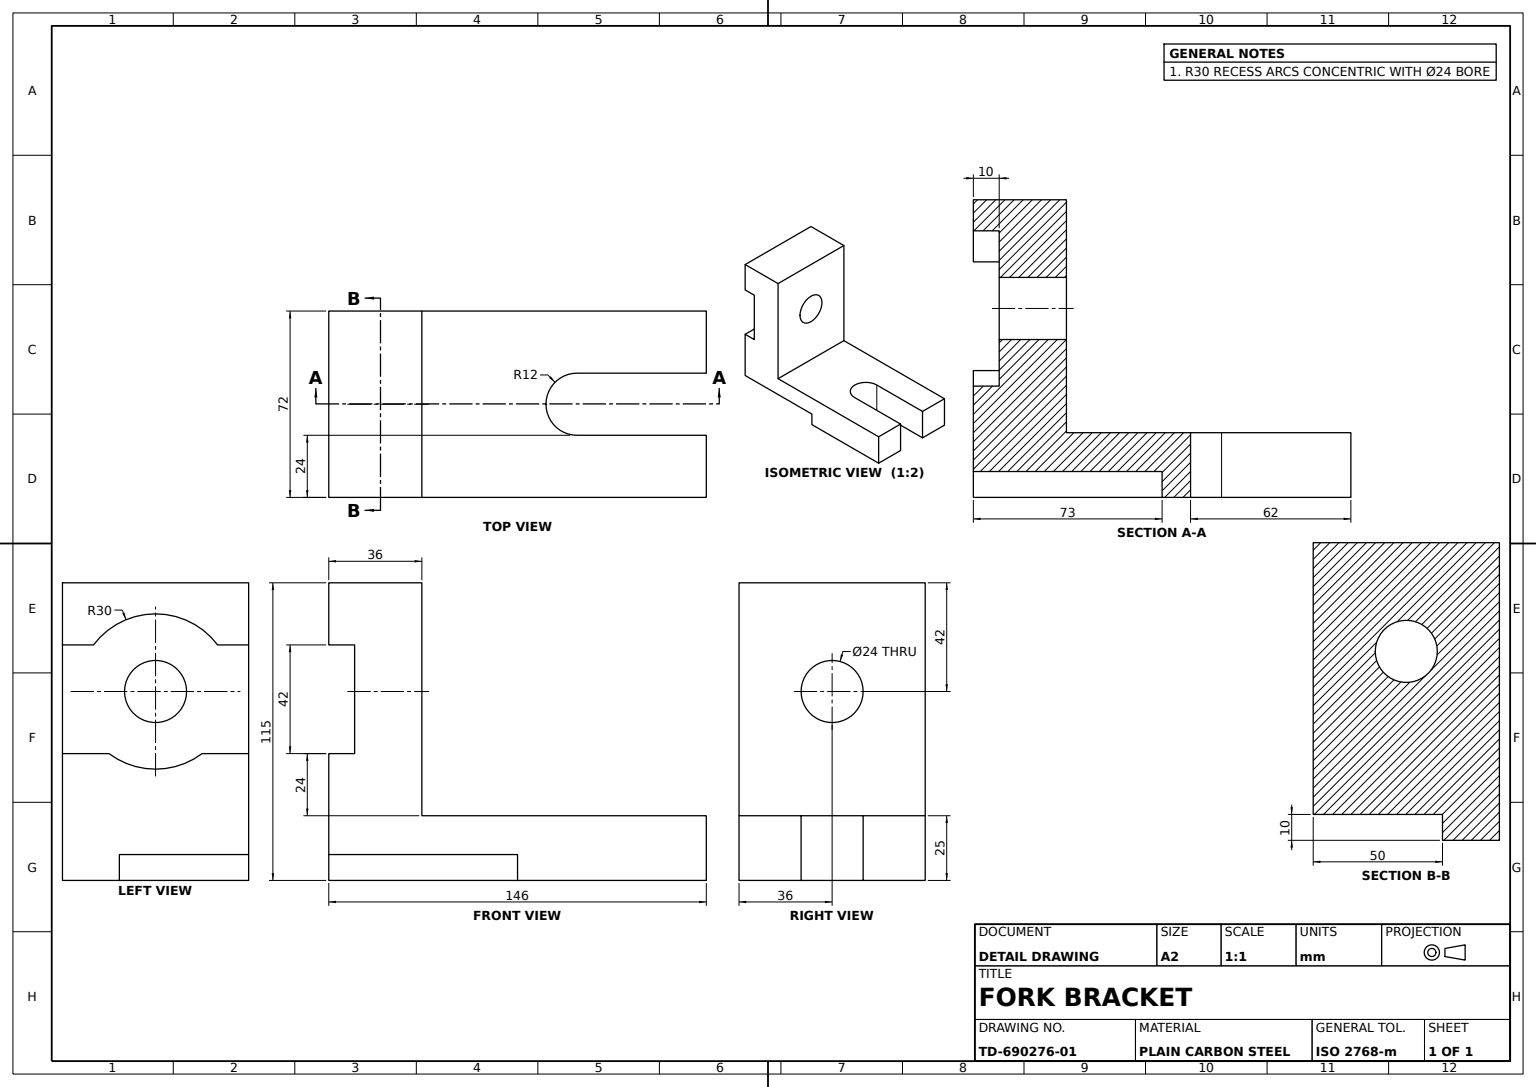
from build123d import *

# Parameters (mm, degrees)
UPRIGHT_BLOCK_PROFILE_W             = 72
UPRIGHT_BLOCK_PROFILE_H             = 90
UPRIGHT_BLOCK_DEPTH                 = 36
SIDE_RECESS_10_DEEP_DEPTH           = 10
BORE_SKETCH_R                       = 12
BORE_24_DEPTH                       = 42
BASE_ARM_SKETCH_W                   = 146
BASE_ARM_SKETCH_H                   = 25
BASE_ARM_146X25_DEPTH               = 72
ARM_SLOT_DEPTH                      = 42
RELIEF_GROOVE_SKETCH_W              = 50
RELIEF_GROOVE_SKETCH_H              = 10
UNDERSIDE_RELIEF_GROOVE_10X50_DEPTH = 73


with BuildPart() as part:
    # Upright Block Profile → Upright Block (new body)
    with BuildSketch(Plane.XY):
        with Locations((36, 45)):
            Rectangle(UPRIGHT_BLOCK_PROFILE_W, UPRIGHT_BLOCK_PROFILE_H)
    extrude(amount=-UPRIGHT_BLOCK_DEPTH)

    # Side Recess Sketch → Side Recess 10 Deep (cut)
    with BuildSketch(Plane.XY):
        with BuildLine():
            Line((0, 66), (12, 66))
            ThreePointArc((12, 66), (36, 78), (60, 66))
            Line((60, 66), (72, 66))
            Line((72, 66), (72, 24))
            Line((72, 24), (54, 24))
            ThreePointArc((54, 24), (36, 18), (18, 24))
            Line((18, 24), (0, 24))
            Line((0, 24), (0, 66))
        make_face()
    extrude(amount=-SIDE_RECESS_10_DEEP_DEPTH, mode=Mode.SUBTRACT)

    # Bore Sketch → Bore Ø24 (cut)
    with BuildSketch(Plane.XY.offset(-10)):
        with Locations((36, 48)):
            Circle(BORE_SKETCH_R)
    extrude(amount=-BORE_24_DEPTH, mode=Mode.SUBTRACT)

    # Base Arm Sketch → Base Arm 146x25 (add)
    with BuildSketch(Plane(origin=(72, 0, 0), x_dir=(0, 0, -1), z_dir=(1, 0, 0))):
        with Locations((73, -12.5)):
            Rectangle(BASE_ARM_SKETCH_W, BASE_ARM_SKETCH_H)
    extrude(amount=-BASE_ARM_146X25_DEPTH)

    # Arm Slot Sketch → Arm Slot (cut)
    with BuildSketch(Plane(origin=(0, 0, 0), x_dir=(1, 0, 0), z_dir=(0, 1, 0))):
        with BuildLine():
            Line((24, 146), (24, 96))
            ThreePointArc((24, 96), (36, 84), (48, 96))
            Line((48, 96), (48, 146))
            Line((48, 146), (24, 146))
        make_face()
    extrude(amount=-ARM_SLOT_DEPTH, mode=Mode.SUBTRACT)

    # Relief Groove Sketch → Underside Relief Groove 10x50 (cut)
    with BuildSketch(Plane.XY):
        with Locations((47, -20)):
            Rectangle(RELIEF_GROOVE_SKETCH_W, RELIEF_GROOVE_SKETCH_H)
    extrude(amount=-UNDERSIDE_RELIEF_GROOVE_10X50_DEPTH, mode=Mode.SUBTRACT)


solid = part.part
